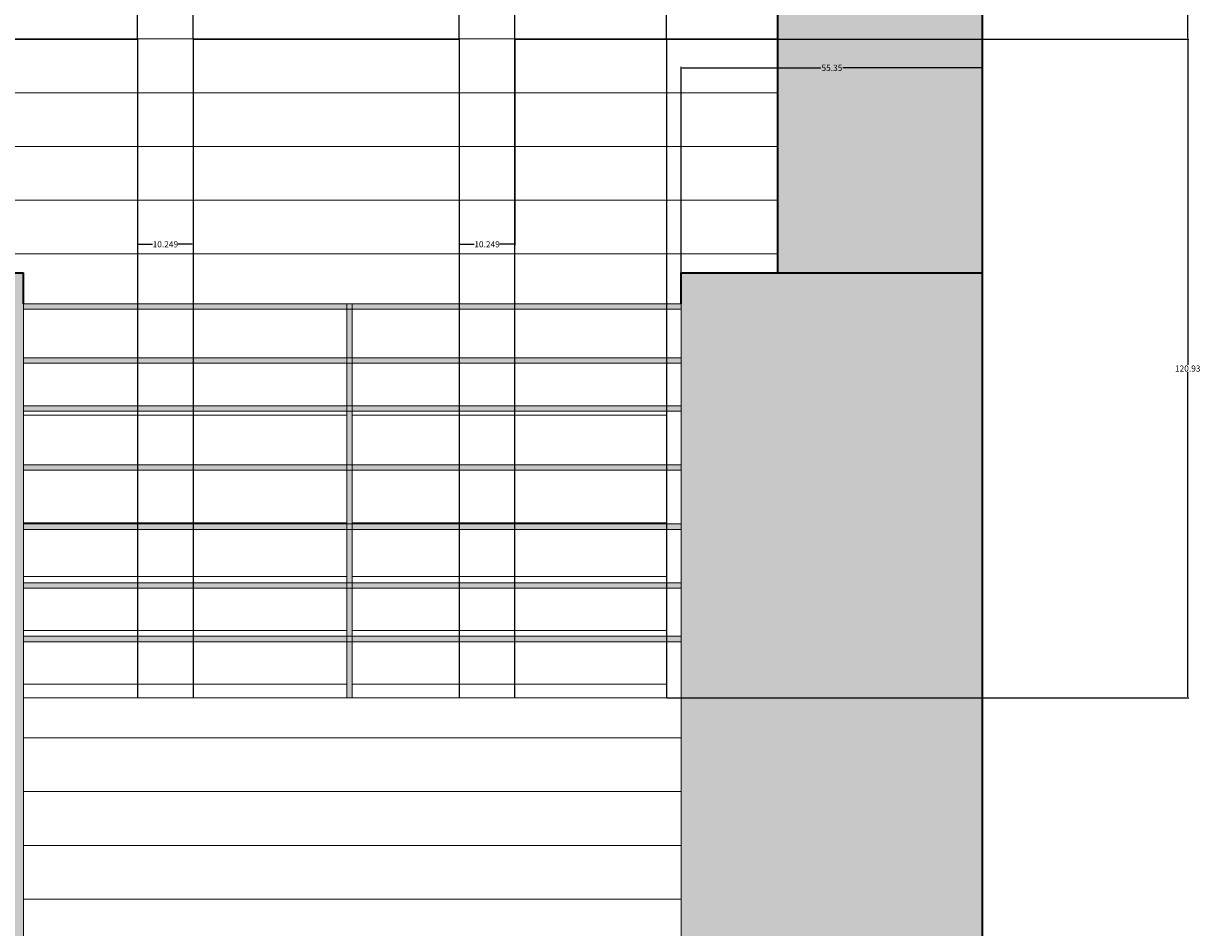
# Model space of a CAD drawing. Units: inches. Extents: x 8 to 634, y 41 to 867.
# Tile 20 of 21: x 418 to 634, y 577 to 743. Entities that reach past the tile are written whole.
import ezdxf

# ---------------------------------------------------------------- set-up
doc = ezdxf.new("R2010")
doc.units = ezdxf.units.IN
doc.header["$MEASUREMENT"] = 0
for name, color, linetype, lineweight in [('A-ANNO-DIMS', 2, 'Continuous', 18), ('A-FLOR-HRAL', 7, 'Continuous', 18), ('A-FLOR-HRAL-PATT', 252, 'Continuous', 9), ('A-GLAZ', 4, 'Continuous', 25), ('A-ROOF', 7, 'Continuous', 35), ('A-ROOF-PATT', 8, 'Continuous', 9), ('A-WALL', 7, 'Continuous', 35), ('A-WALL-PANL', 7, 'Continuous', 18), ('A-WALL-PATT', 8, 'Continuous', 9)]:
    doc.layers.add(name, color=color, linetype=linetype, lineweight=lineweight)
doc.layers.add('A-GLAZ-PATT', color=251, linetype='Continuous', lineweight=9, true_color=0x636466)
doc.styles.get("Standard").update_dxf_attribs({"font": 'arial.ttf'})
doc.dimstyles.get("Standard").update_dxf_attribs({"dimtxt": 1.125, "dimasz": 0.18, "dimexe": 0.18, "dimexo": 0.0625, "dimgap": 0.09, "dimtad": 0, "dimtih": 1, "dimtoh": 1, "dimdec": 4, "dimzin": 0, "dimdsep": 46, "dimlunit": 4, "dimtxsty": 'Standard', "dimcen": 0.09, "dimadec": 0, "dimazin": 0, "dimtfac": 1, "dimtdec": 4, "dimtofl": 0, "dimtmove": 0, "dimatfit": 3, "dimfxl": 1, "dimtolj": 1, "dimtzin": 0, "dimarcsym": 0})

# ---------------------------------------------------------------- blocks, each defined once
blk = doc.blocks.new('*D19')
at = {"layer": 'A-ANNO-DIMS', "color": 0, "lineweight": -2, "transparency": 16777216}
for p, q in [((47.34, 697.73), (47.34, 866.81)), ((47.52, 866.63), (319.51, 866.63)), ((594.17, 866.63), (322.18, 866.63)), ((594.35, 827.83), (594.35, 866.81))]:
    blk.add_line(p, q, dxfattribs=at)
at = {"layer": 'A-ANNO-DIMS', "color": 0, "transparency": 16777216}
for points in [[(47.52, 866.66), (47.52, 866.6), (47.34, 866.63)], [(594.17, 866.66), (594.17, 866.6), (594.35, 866.63)]]:
    blk.add_solid(points, dxfattribs=at)
at = {"layer": 'Defpoints', "color": 0, "transparency": 16777216}
for p in [(594.35, 866.63), (594.35, 827.77), (47.34, 697.67)]:
    blk.add_point(p, dxfattribs=at)
at = {"layer": 'A-ANNO-DIMS', "color": 0, "transparency": 16777216, "insert": (320.85, 866.63), "char_height": 1.125, "attachment_point": 5}
blk.add_mtext('\\A1;547', dxfattribs=at)
blk = doc.blocks.new('*D44')
at = {"layer": 'A-ANNO-DIMS', "color": 0, "lineweight": -2, "transparency": 16777216}
for p, q in [((536.38, 740.56), (632.18, 740.56)), ((632, 740.38), (632, 680.76)), ((632, 619.81), (632, 679.43)), ((536.38, 619.63), (632.18, 619.63))]:
    blk.add_line(p, q, dxfattribs=at)
at = {"layer": 'A-ANNO-DIMS', "color": 0, "transparency": 16777216}
for points in [[(631.97, 740.38), (632.03, 740.38), (632, 740.56)], [(631.97, 619.81), (632.03, 619.81), (632, 619.63)]]:
    blk.add_solid(points, dxfattribs=at)
at = {"layer": 'Defpoints', "color": 0, "transparency": 16777216}
for p in [(536.32, 740.56), (632, 740.56), (536.32, 619.63)]:
    blk.add_point(p, dxfattribs=at)
at = {"layer": 'A-ANNO-DIMS', "color": 0, "transparency": 16777216, "insert": (632, 680.09), "char_height": 1.125, "attachment_point": 5}
blk.add_mtext('\\A1;120.93', dxfattribs=at)
blk = doc.blocks.new('*D45')
at = {"layer": 'A-ANNO-DIMS', "color": 0, "lineweight": -2, "transparency": 16777216}
for p, q in [((556.77, 776.89), (632.18, 776.89)), ((632, 776.71), (632, 759.39)), ((632, 740.74), (632, 758.06)), ((536.38, 740.56), (632.18, 740.56))]:
    blk.add_line(p, q, dxfattribs=at)
at = {"layer": 'A-ANNO-DIMS', "color": 0, "transparency": 16777216}
for points in [[(631.97, 776.71), (632.03, 776.71), (632, 776.89)], [(631.97, 740.74), (632.03, 740.74), (632, 740.56)]]:
    blk.add_solid(points, dxfattribs=at)
at = {"layer": 'Defpoints', "color": 0, "transparency": 16777216}
for p in [(556.71, 776.89), (632, 776.89), (536.32, 740.56)]:
    blk.add_point(p, dxfattribs=at)
at = {"layer": 'A-ANNO-DIMS', "color": 0, "transparency": 16777216, "insert": (632, 758.72), "char_height": 1.125, "attachment_point": 5}
blk.add_mtext('\\A1;36.34', dxfattribs=at)
blk = doc.blocks.new('*D50')
at = {"layer": 'A-ANNO-DIMS', "color": 0, "lineweight": -2, "transparency": 16777216}
for p, q in [((370.39, 740.62), (370.39, 778.39)), ((370.57, 778.21), (402.91, 778.21)), ((439.02, 778.21), (406.68, 778.21)), ((439.2, 740.62), (439.2, 778.39))]:
    blk.add_line(p, q, dxfattribs=at)
at = {"layer": 'A-ANNO-DIMS', "color": 0, "transparency": 16777216}
for points in [[(370.57, 778.24), (370.57, 778.18), (370.39, 778.21)], [(439.02, 778.24), (439.02, 778.18), (439.2, 778.21)]]:
    blk.add_solid(points, dxfattribs=at)
at = {"layer": 'Defpoints', "color": 0, "transparency": 16777216}
for p in [(439.2, 778.21), (370.39, 740.56), (439.2, 740.56)]:
    blk.add_point(p, dxfattribs=at)
at = {"layer": 'A-ANNO-DIMS', "color": 0, "transparency": 16777216, "insert": (404.79, 778.21), "char_height": 1.125, "attachment_point": 5}
blk.add_mtext('\\A1;68.81', dxfattribs=at)
blk = doc.blocks.new('*D51')
at = {"layer": 'A-ANNO-DIMS', "color": 0, "lineweight": -2, "transparency": 16777216}
for p, q in [((439.2, 740.49), (439.2, 702.73)), ((449.45, 740.49), (449.45, 702.73)), ((439.38, 702.91), (441.95, 702.91)), ((449.27, 702.91), (446.7, 702.91))]:
    blk.add_line(p, q, dxfattribs=at)
at = {"layer": 'A-ANNO-DIMS', "color": 0, "transparency": 16777216}
for points in [[(439.38, 702.94), (439.38, 702.88), (439.2, 702.91)], [(449.27, 702.94), (449.27, 702.88), (449.45, 702.91)]]:
    blk.add_solid(points, dxfattribs=at)
at = {"layer": 'Defpoints', "color": 0, "transparency": 16777216}
for p in [(439.2, 740.56), (449.45, 740.56), (439.2, 702.91)]:
    blk.add_point(p, dxfattribs=at)
at = {"layer": 'A-ANNO-DIMS', "color": 0, "transparency": 16777216, "insert": (444.33, 702.91), "char_height": 1.125, "attachment_point": 5}
blk.add_mtext('\\A1;10.249', dxfattribs=at)
blk = doc.blocks.new('*D52')
at = {"layer": 'A-ANNO-DIMS', "color": 0, "lineweight": -2, "transparency": 16777216}
for p, q in [((449.45, 740.62), (449.45, 778.39)), ((449.63, 778.21), (472.28, 778.21)), ((498.07, 778.21), (475.43, 778.21)), ((498.25, 740.62), (498.25, 778.39))]:
    blk.add_line(p, q, dxfattribs=at)
at = {"layer": 'A-ANNO-DIMS', "color": 0, "transparency": 16777216}
for points in [[(449.63, 778.24), (449.63, 778.18), (449.45, 778.21)], [(498.07, 778.24), (498.07, 778.18), (498.25, 778.21)]]:
    blk.add_solid(points, dxfattribs=at)
at = {"layer": 'Defpoints', "color": 0, "transparency": 16777216}
for p in [(498.25, 778.21), (449.45, 740.56), (498.25, 740.56)]:
    blk.add_point(p, dxfattribs=at)
at = {"layer": 'A-ANNO-DIMS', "color": 0, "transparency": 16777216, "insert": (473.85, 778.21), "char_height": 1.125, "attachment_point": 5}
blk.add_mtext('\\A1;48.8', dxfattribs=at)
blk = doc.blocks.new('*D53')
at = {"layer": 'A-ANNO-DIMS', "color": 0, "lineweight": -2, "transparency": 16777216}
for p, q in [((498.25, 740.49), (498.25, 702.73)), ((508.5, 740.49), (508.5, 702.73)), ((498.43, 702.91), (501, 702.91)), ((508.32, 702.91), (505.75, 702.91))]:
    blk.add_line(p, q, dxfattribs=at)
at = {"layer": 'A-ANNO-DIMS', "color": 0, "transparency": 16777216}
for points in [[(498.43, 702.94), (498.43, 702.88), (498.25, 702.91)], [(508.32, 702.94), (508.32, 702.88), (508.5, 702.91)]]:
    blk.add_solid(points, dxfattribs=at)
at = {"layer": 'Defpoints', "color": 0, "transparency": 16777216}
for p in [(498.25, 740.56), (508.5, 740.56), (498.25, 702.91)]:
    blk.add_point(p, dxfattribs=at)
at = {"layer": 'A-ANNO-DIMS', "color": 0, "transparency": 16777216, "insert": (503.38, 702.91), "char_height": 1.125, "attachment_point": 5}
blk.add_mtext('\\A1;10.249', dxfattribs=at)
blk = doc.blocks.new('*D54')
at = {"layer": 'A-ANNO-DIMS', "color": 0, "lineweight": -2, "transparency": 16777216}
for p, q in [((508.5, 740.62), (508.5, 778.39)), ((508.68, 778.21), (520.42, 778.21)), ((536.14, 778.21), (524.4, 778.21)), ((536.32, 740.62), (536.32, 778.39))]:
    blk.add_line(p, q, dxfattribs=at)
at = {"layer": 'A-ANNO-DIMS', "color": 0, "transparency": 16777216}
for points in [[(508.68, 778.24), (508.68, 778.18), (508.5, 778.21)], [(536.14, 778.24), (536.14, 778.18), (536.32, 778.21)]]:
    blk.add_solid(points, dxfattribs=at)
at = {"layer": 'Defpoints', "color": 0, "transparency": 16777216}
for p in [(536.32, 778.21), (508.5, 740.56), (536.32, 740.56)]:
    blk.add_point(p, dxfattribs=at)
at = {"layer": 'A-ANNO-DIMS', "color": 0, "transparency": 16777216, "insert": (522.41, 778.21), "char_height": 1.125, "attachment_point": 5}
blk.add_mtext('\\A1;27.82', dxfattribs=at)
blk = doc.blocks.new('*D56')
at = {"layer": 'A-ANNO-DIMS', "color": 0, "lineweight": -2, "transparency": 16777216}
for p, q in [((539, 697.73), (539, 735.5)), ((539.18, 735.32), (564.68, 735.32)), ((594.17, 735.32), (568.67, 735.32)), ((594.35, 697.73), (594.35, 735.5))]:
    blk.add_line(p, q, dxfattribs=at)
at = {"layer": 'A-ANNO-DIMS', "color": 0, "transparency": 16777216}
for points in [[(539.18, 735.35), (539.18, 735.29), (539, 735.32)], [(594.17, 735.35), (594.17, 735.29), (594.35, 735.32)]]:
    blk.add_solid(points, dxfattribs=at)
at = {"layer": 'Defpoints', "color": 0, "transparency": 16777216}
for p in [(594.35, 735.32), (539, 697.67), (594.35, 697.67)]:
    blk.add_point(p, dxfattribs=at)
at = {"layer": 'A-ANNO-DIMS', "color": 0, "transparency": 16777216, "insert": (566.68, 735.32), "char_height": 1.125, "attachment_point": 5}
blk.add_mtext('\\A1;55.35', dxfattribs=at)

msp = doc.modelspace()

# ---------------------------------------------------------------- hatches: boundary and pattern name
at = {"layer": 'A-FLOR-HRAL-PATT', "transparency": 33554687}
h = msp.add_hatch(color=256, dxfattribs=at)
h.dxf.hatch_style = 1
h.paths.add_polyline_path([(439.201, 691.978), (418.2881, 691.978), (418.2881, 690.978), (439.201, 690.978)])
h.paths.add_polyline_path([(449.4498, 691.978), (439.201, 691.978), (439.201, 690.978), (449.4498, 690.978)])
h.paths.add_polyline_path([(477.6441, 691.978), (449.4498, 691.978), (449.4498, 690.978), (477.6441, 690.978)])
h.paths.add_polyline_path([(477.6441, 682.0586), (449.4498, 682.0586), (449.4498, 681.0586), (477.6441, 681.0586)])
h.paths.add_polyline_path([(449.4498, 682.0586), (439.201, 682.0586), (439.201, 681.0586), (449.4498, 681.0586)])
h.paths.add_polyline_path([(439.201, 682.0586), (418.2881, 682.0586), (418.2881, 681.0586), (439.201, 681.0586)])
h.paths.add_polyline_path([(439.201, 673.2414), (418.2881, 673.2414), (418.2881, 672.2414), (439.201, 672.2414)])
h.paths.add_polyline_path([(449.4498, 673.2414), (439.201, 673.2414), (439.201, 672.2414), (449.4498, 672.2414)])
h.paths.add_polyline_path([(539.0002, 673.2414), (449.4498, 673.2414), (449.4498, 672.2414), (539.0002, 672.2414)])
h.paths.add_polyline_path([(439.201, 662.4168), (418.2881, 662.4168), (418.2881, 661.4168), (439.201, 661.4168)], flags=16)
h.paths.add_polyline_path([(449.4498, 662.4168), (439.201, 662.4168), (439.201, 661.4168), (449.4498, 661.4168)], flags=16)
h.paths.add_polyline_path([(477.6441, 662.4168), (449.4498, 662.4168), (449.4498, 661.4168), (477.6441, 661.4168)], flags=16)
h.paths.add_polyline_path([(439.201, 651.537), (418.2881, 651.537), (418.2881, 650.537), (439.201, 650.537)])
h.paths.add_polyline_path([(449.4498, 651.537), (439.201, 651.537), (439.201, 650.537), (449.4498, 650.537)])
h.paths.add_polyline_path([(477.6441, 651.537), (449.4498, 651.537), (449.4498, 650.537), (477.6441, 650.537)])
h.paths.add_polyline_path([(439.201, 640.7358), (418.2881, 640.7358), (418.2881, 639.7358), (439.201, 639.7358)])
h.paths.add_polyline_path([(449.4498, 640.7358), (439.201, 640.7358), (439.201, 639.7358), (449.4498, 639.7358)])
h.paths.add_polyline_path([(477.6441, 640.7358), (449.4498, 640.7358), (449.4498, 639.7358), (477.6441, 639.7358)])
h.paths.add_polyline_path([(439.201, 630.9186), (418.2881, 630.9186), (418.2881, 629.9186), (439.201, 629.9186)])
h.paths.add_polyline_path([(449.4498, 630.9186), (439.201, 630.9186), (439.201, 629.9186), (449.4498, 629.9186)])
h.paths.add_polyline_path([(477.6441, 630.9186), (449.4498, 630.9186), (449.4498, 629.9186), (477.6441, 629.9186)])
h.paths.add_polyline_path([(498.2535, 630.9186), (478.6441, 630.9186), (478.6441, 629.9186), (498.2535, 629.9186)])
h.paths.add_polyline_path([(478.6441, 639.7358), (477.6441, 639.7358), (477.6441, 630.9186), (478.6441, 630.9186)])
h.paths.add_polyline_path([(478.6441, 630.9186), (477.6441, 630.9186), (477.6441, 629.9186), (478.6441, 629.9186)])
h.paths.add_polyline_path([(478.6441, 629.9186), (477.6441, 629.9186), (477.6441, 619.6298), (478.6441, 619.6298)])
h.paths.add_polyline_path([(508.5023, 630.9186), (498.2535, 630.9186), (498.2535, 629.9186), (508.5023, 629.9186)])
h.paths.add_polyline_path([(536.3204, 630.9186), (508.5023, 630.9186), (508.5023, 629.9186), (536.3204, 629.9186)])
h.paths.add_polyline_path([(539.0002, 630.9186), (536.3204, 630.9186), (536.3204, 629.9186), (539.0002, 629.9186)])
h.paths.add_polyline_path([(539.0002, 640.7358), (536.3204, 640.7358), (536.3204, 639.7358), (539.0002, 639.7358)])
h.paths.add_polyline_path([(536.3204, 640.7358), (508.5023, 640.7358), (508.5023, 639.7358), (536.3204, 639.7358)])
h.paths.add_polyline_path([(508.5023, 640.7358), (498.2535, 640.7358), (498.2535, 639.7358), (508.5023, 639.7358)])
h.paths.add_polyline_path([(498.2535, 640.7358), (478.6441, 640.7358), (478.6441, 639.7358), (498.2535, 639.7358)])
h.paths.add_polyline_path([(498.2535, 651.537), (478.6441, 651.537), (478.6441, 650.537), (498.2535, 650.537)])
h.paths.add_polyline_path([(478.6441, 651.537), (477.6441, 651.537), (477.6441, 650.537), (478.6441, 650.537)])
h.paths.add_polyline_path([(478.6441, 661.4168), (477.6441, 661.4168), (477.6441, 651.537), (478.6441, 651.537)])
h.paths.add_polyline_path([(478.6441, 650.537), (477.6441, 650.537), (477.6441, 640.7358), (478.6441, 640.7358)])
h.paths.add_polyline_path([(478.6441, 640.7358), (477.6441, 640.7358), (477.6441, 639.7358), (478.6441, 639.7358)])
h.paths.add_polyline_path([(508.5023, 651.537), (498.2535, 651.537), (498.2535, 650.537), (508.5023, 650.537)])
h.paths.add_polyline_path([(536.3204, 651.537), (508.5023, 651.537), (508.5023, 650.537), (536.3204, 650.537)])
h.paths.add_polyline_path([(539.0002, 651.537), (536.3204, 651.537), (536.3204, 650.537), (539.0002, 650.537)])
h.paths.add_polyline_path([(539.0002, 662.4168), (536.3204, 662.4168), (536.3204, 661.4168), (539.0002, 661.4168)])
h.paths.add_polyline_path([(536.3204, 662.4168), (508.5023, 662.4168), (508.5023, 661.4168), (536.3204, 661.4168)])
h.paths.add_polyline_path([(508.5023, 662.4168), (498.2535, 662.4168), (498.2535, 661.4168), (508.5023, 661.4168)])
h.paths.add_polyline_path([(498.2535, 662.4168), (418.2881, 662.4168), (418.2881, 661.4168), (498.2535, 661.4168)])
h.paths.add_polyline_path([(478.6441, 672.2414), (477.6441, 672.2414), (477.6441, 662.4168), (478.6441, 662.4168)])
h.paths.add_polyline_path([(478.6441, 681.0586), (477.6441, 681.0586), (477.6441, 673.2414), (478.6441, 673.2414)])
h = msp.add_hatch(color=256, dxfattribs=at)
h.dxf.hatch_style = 1
h.paths.add_polyline_path([(498.2535, 682.0586), (478.6441, 682.0586), (478.6441, 681.0586), (498.2535, 681.0586)])
h.paths.add_polyline_path([(508.5023, 682.0586), (498.2535, 682.0586), (498.2535, 681.0586), (508.5023, 681.0586)])
h.paths.add_polyline_path([(536.3204, 682.0586), (508.5023, 682.0586), (508.5023, 681.0586), (536.3204, 681.0586)])
h.paths.add_polyline_path([(478.6441, 690.978), (477.6441, 690.978), (477.6441, 682.0586), (478.6441, 682.0586)])
h.paths.add_polyline_path([(478.6441, 682.0586), (477.6441, 682.0586), (477.6441, 681.0586), (478.6441, 681.0586)])
h.paths.add_polyline_path([(477.6441, 662.4168), (449.4498, 662.4168), (449.4498, 661.4168), (477.6441, 661.4168)])
h.paths.add_polyline_path([(449.4498, 662.4168), (439.201, 662.4168), (439.201, 661.4168), (449.4498, 661.4168)])
h.paths.add_polyline_path([(439.201, 662.4168), (418.2881, 662.4168), (418.2881, 661.4168), (439.201, 661.4168)])
h.paths.add_polyline_path([(478.6441, 691.978), (477.6441, 691.978), (477.6441, 690.978), (478.6441, 690.978)])
h.paths.add_polyline_path([(498.2535, 691.978), (478.6441, 691.978), (478.6441, 690.978), (498.2535, 690.978)])
h.paths.add_polyline_path([(508.5023, 691.978), (498.2535, 691.978), (498.2535, 690.978), (508.5023, 690.978)])
h.paths.add_polyline_path([(536.3204, 691.978), (508.5023, 691.978), (508.5023, 690.978), (536.3204, 690.978)])
h.paths.add_polyline_path([(539.0002, 691.978), (536.3204, 691.978), (536.3204, 690.978), (539.0002, 690.978)])
h.paths.add_polyline_path([(539.0002, 682.0586), (536.3204, 682.0586), (536.3204, 681.0586), (539.0002, 681.0586)])
at = {"layer": 'A-GLAZ-PATT', "transparency": 33554687}
h = msp.add_hatch(dxfattribs=at)
h.set_pattern_fill('ANSI31', color=256, scale=79, angle=135)
h.paths.add_polyline_path([(355.7466, 740.5561), (322.56, 740.5561), (322.56, 697.6655), (355.7466, 697.6655)])
h.paths.add_polyline_path([(439.201, 740.5561), (370.3877, 740.5561), (370.3877, 697.6655), (418.2881, 697.6655), (418.2881, 691.978), (439.201, 691.978)])
h.paths.add_polyline_path([(498.2535, 740.5561), (449.4498, 740.5561), (449.4498, 691.978), (498.2535, 691.978)])
h.paths.add_polyline_path([(536.3204, 740.5561), (508.5023, 740.5561), (508.5023, 691.978), (536.3204, 691.978)])
h.paths.add_polyline_path([(439.201, 690.978), (418.2881, 690.978), (418.2881, 682.0586), (439.201, 682.0586)])
h.paths.add_polyline_path([(439.201, 681.0586), (418.2881, 681.0586), (418.2881, 673.2414), (439.201, 673.2414)])
h.paths.add_polyline_path([(439.201, 672.2414), (418.2881, 672.2414), (418.2881, 662.4168), (439.201, 662.4168)])
h.paths.add_polyline_path([(439.201, 661.4168), (418.2881, 661.4168), (418.2881, 651.537), (439.201, 651.537)])
h.paths.add_polyline_path([(439.201, 650.537), (418.2881, 650.537), (418.2881, 640.7358), (439.201, 640.7358)])
h.paths.add_polyline_path([(439.201, 639.7358), (418.2881, 639.7358), (418.2881, 630.9186), (439.201, 630.9186)])
h.paths.add_polyline_path([(439.201, 629.9186), (418.2881, 629.9186), (418.2881, 619.6298), (439.201, 619.6298)])
h.paths.add_polyline_path([(477.6441, 629.9186), (449.4498, 629.9186), (449.4498, 619.6298), (477.6441, 619.6298)])
h.paths.add_polyline_path([(477.6441, 639.7358), (449.4498, 639.7358), (449.4498, 630.9186), (477.6441, 630.9186)])
h.paths.add_polyline_path([(477.6441, 650.537), (449.4498, 650.537), (449.4498, 640.7358), (477.6441, 640.7358)])
h.paths.add_polyline_path([(477.6441, 661.4168), (449.4498, 661.4168), (449.4498, 651.537), (477.6441, 651.537)])
h.paths.add_polyline_path([(477.6441, 672.2414), (449.4498, 672.2414), (449.4498, 662.4168), (477.6441, 662.4168)])
h.paths.add_polyline_path([(477.6441, 681.0586), (449.4498, 681.0586), (449.4498, 673.2414), (477.6441, 673.2414)])
h.paths.add_polyline_path([(477.6441, 690.978), (449.4498, 690.978), (449.4498, 682.0586), (477.6441, 682.0586)])
h.paths.add_polyline_path([(498.2535, 690.978), (478.6441, 690.978), (478.6441, 682.0586), (498.2535, 682.0586)])
h.paths.add_polyline_path([(498.2535, 681.0586), (478.6441, 681.0586), (478.6441, 673.2414), (498.2535, 673.2414)])
h.paths.add_polyline_path([(498.2535, 672.2414), (478.6441, 672.2414), (478.6441, 662.4168), (498.2535, 662.4168)])
h.paths.add_polyline_path([(498.2535, 661.4168), (478.6441, 661.4168), (478.6441, 651.537), (498.2535, 651.537)])
h.paths.add_polyline_path([(498.2535, 650.537), (478.6441, 650.537), (478.6441, 640.7358), (498.2535, 640.7358)])
h.paths.add_polyline_path([(498.2535, 639.7358), (478.6441, 639.7358), (478.6441, 630.9186), (498.2535, 630.9186)])
h.paths.add_polyline_path([(498.2535, 629.9186), (478.6441, 629.9186), (478.6441, 619.6298), (498.2535, 619.6298)])
h.paths.add_polyline_path([(536.3204, 629.9186), (508.5023, 629.9186), (508.5023, 619.6298), (536.3204, 619.6298)])
h.paths.add_polyline_path([(536.3204, 639.7358), (508.5023, 639.7358), (508.5023, 630.9186), (536.3204, 630.9186)])
h.paths.add_polyline_path([(536.3204, 650.537), (508.5023, 650.537), (508.5023, 640.7358), (536.3204, 640.7358)])
h.paths.add_polyline_path([(536.3204, 661.4168), (508.5023, 661.4168), (508.5023, 651.537), (536.3204, 651.537)])
h.paths.add_polyline_path([(536.3204, 672.2414), (508.5023, 672.2414), (508.5023, 662.4168), (536.3204, 662.4168)])
h.paths.add_polyline_path([(536.3204, 681.0586), (508.5023, 681.0586), (508.5023, 673.2414), (536.3204, 673.2414)])
h.paths.add_polyline_path([(536.3204, 690.978), (508.5023, 690.978), (508.5023, 682.0586), (536.3204, 682.0586)])
h.paths.add_polyline_path([(342.6544, 175.7749), (302.6522, 224.3257), (302.6522, 101.0012), (342.6544, 149.552)])
h.paths.add_polyline_path([(342.6544, 224.3257), (302.6522, 224.3257), (342.6544, 175.7749)])
h.paths.add_polyline_path([(342.6544, 149.552), (302.6522, 101.0012), (342.6544, 101.0012)])
h.paths.add_polyline_path([(353.4573, 162.6634), (342.6544, 149.552), (342.6544, 101.0012), (353.4573, 101.0012)])
h.paths.add_polyline_path([(353.4573, 224.3257), (342.6544, 224.3257), (342.6544, 101.0012), (353.4573, 101.0012)])
h.paths.add_polyline_path([(342.6544, 175.7749), (342.6544, 149.552), (353.4573, 162.6634)], flags=17)
h = msp.add_hatch(dxfattribs=at)
h.set_pattern_fill('ANSI31', color=256, scale=79, angle=135)
h.paths.add_polyline_path([(449.4498, 690.978), (439.201, 690.978), (439.201, 682.0586), (449.4498, 682.0586)])
h.paths.add_polyline_path([(449.4498, 681.0586), (439.201, 681.0586), (439.201, 673.2414), (449.4498, 673.2414)])
h.paths.add_polyline_path([(449.4498, 672.2414), (439.201, 672.2414), (439.201, 662.4168), (449.4498, 662.4168)])
h.paths.add_polyline_path([(449.4498, 661.4168), (439.201, 661.4168), (439.201, 651.537), (449.4498, 651.537)])
h.paths.add_polyline_path([(449.4498, 650.537), (439.201, 650.537), (439.201, 640.7358), (449.4498, 640.7358)])
h.paths.add_polyline_path([(449.4498, 639.7358), (439.201, 639.7358), (439.201, 630.9186), (449.4498, 630.9186)])
h.paths.add_polyline_path([(449.4498, 629.9186), (439.201, 629.9186), (439.201, 619.6298), (449.4498, 619.6298)])
h.paths.add_polyline_path([(508.5023, 629.9186), (498.2535, 629.9186), (498.2535, 619.6298), (508.5023, 619.6298)])
h.paths.add_polyline_path([(508.5023, 639.7358), (498.2535, 639.7358), (498.2535, 630.9186), (508.5023, 630.9186)])
h.paths.add_polyline_path([(508.5023, 650.537), (498.2535, 650.537), (498.2535, 640.7358), (508.5023, 640.7358)])
h.paths.add_polyline_path([(508.5023, 661.4168), (498.2535, 661.4168), (498.2535, 651.537), (508.5023, 651.537)])
h.paths.add_polyline_path([(508.5023, 672.2414), (498.2535, 672.2414), (498.2535, 662.4168), (508.5023, 662.4168)])
h.paths.add_polyline_path([(508.5023, 681.0586), (498.2535, 681.0586), (498.2535, 673.2414), (508.5023, 673.2414)])
h.paths.add_polyline_path([(508.5023, 690.978), (498.2535, 690.978), (498.2535, 682.0586), (508.5023, 682.0586)])
at = {"layer": 'A-ROOF-PATT', "transparency": 33554687}
h = msp.add_hatch(dxfattribs=at)
h.set_pattern_fill('AR-CONC', color=256, scale=2.2, angle=135)
h.paths.add_polyline_path([(262.2266, 828.9821), (144.3564, 828.9821), (144.3564, 697.6655), (262.2266, 785.231), (245.114, 785.231), (245.114, 792.8938), (262.2266, 792.8938)])
h.paths.add_polyline_path([(594.3501, 827.7671), (262.2266, 827.7671), (262.2266, 792.8938), (262.2266, 697.6655), (299.7961, 697.6655), (299.7961, 776.8929), (556.7072, 776.8929), (556.7072, 774.3342), (556.7072, 697.6655), (594.3501, 697.6655)])
at = {"layer": 'A-WALL-PATT', "transparency": 33554687}
h = msp.add_hatch(dxfattribs=at)
h.set_pattern_fill('ANSI31', color=256, scale=79, angle=135)
h.paths.add_polyline_path([(539.0002, 276.166), (499.4677, 276.166), (418.2881, 276.166), (418.2881, 228.4951), (435.5682, 228.4951), (539.0002, 228.4951)])
h.paths.add_polyline_path([(539.0002, 228.4951), (435.5682, 228.4951), (418.2881, 228.4951), (418.2881, 112.2342), (439.3242, 112.2342), (539.0002, 112.2342)])
h.paths.add_polyline_path([(518.1129, 124.2342), (473.3277, 124.2342), (473.3277, 216.4951), (518.1129, 216.4951)], flags=16)
h.paths.add_polyline_path([(451.2116, 124.2342), (427.4368, 124.2342), (427.4368, 216.4951), (451.2116, 216.4951)], flags=16)
h.paths.add_polyline_path([(539.0002, 112.2342), (439.3242, 112.2342), (418.2881, 112.2342), (418.2881, 91.5417), (539.0002, 91.5417)])
h.paths.add_polyline_path([(539.0002, 392.4268), (427.4368, 392.4268), (418.2881, 392.4268), (418.2881, 391.7598), (418.2881, 276.166), (499.4677, 276.166), (539.0002, 276.166)])
h.paths.add_polyline_path([(518.1129, 288.166), (473.3277, 288.166), (473.3277, 380.4268), (518.1129, 380.4268)], flags=16)
h.paths.add_polyline_path([(451.2116, 288.166), (427.4368, 288.166), (427.4368, 380.4268), (451.2116, 380.4268)], flags=16)
h.paths.add_polyline_path([(539.0002, 451.6305), (427.4368, 452.9097), (418.2881, 452.9097), (418.2881, 392.4268), (427.4368, 392.4268), (539.0002, 392.4268)])
h.paths.add_polyline_path([(539.0002, 569.1705), (427.4368, 569.1705), (418.2881, 569.1705), (418.2881, 452.9097), (427.4368, 452.9097), (539.0002, 451.6305)])
h.paths.add_polyline_path([(473.3277, 557.1705), (518.1129, 557.1705), (518.1129, 464.9097), (473.3277, 464.9097)], flags=16)
h.paths.add_polyline_path([(451.2116, 557.1705), (451.2116, 464.9097), (427.4368, 464.9097), (427.4368, 557.1705)], flags=16)
h.paths.add_polyline_path([(539.0002, 619.6298), (418.2881, 619.6298), (418.2881, 569.1705), (427.4368, 569.1705), (539.0002, 569.1705)])
h.paths.add_polyline_path([(556.7072, 774.3342), (556.7072, 776.8929), (299.7961, 776.8929), (299.7961, 697.6655), (322.56, 697.6655), (322.56, 740.5561), (355.7466, 740.5561), (355.7466, 697.6655), (360.785, 697.6655), (370.3877, 697.6655), (370.3877, 740.5561), (439.201, 740.5561), (439.201, 691.978), (449.4498, 691.978), (449.4498, 740.5561), (498.2535, 740.5561), (498.2535, 691.978), (508.5023, 691.978), (508.5023, 740.5561), (536.3204, 740.5561), (536.3204, 691.978), (539.0002, 691.978), (539.0002, 697.6655), (556.7072, 697.6655)])
h = msp.add_hatch(dxfattribs=at)
h.set_pattern_fill('AR-CONC', color=256, scale=3.2)
h.paths.add_polyline_path([(119.7065, 697.6655), (47.3401, 697.6655), (47.3401, 569.1705), (119.7065, 569.1705)])
h.paths.add_polyline_path([(202.1558, 697.6655), (119.7065, 697.6655), (119.7065, 569.1705), (202.1558, 569.1705)])
h.paths.add_polyline_path([(284.6051, 697.6655), (202.1558, 697.6655), (202.1558, 569.1705), (284.6051, 569.1705)])
h.paths.add_polyline_path([(119.7065, 569.1705), (47.3401, 569.1705), (47.3401, 523.5555), (47.3401, 449.7533), (119.7065, 449.7533)])
h.paths.add_polyline_path([(342.6544, 682.1444), (360.785, 697.6655), (284.6051, 697.6655), (284.6051, 569.1705), (342.6544, 569.1705)])
h.paths.add_polyline_path([(342.6544, 569.1705), (284.6051, 569.1705), (284.6051, 449.7533), (342.6544, 449.7533)])
h.paths.add_polyline_path([(418.2881, 691.978), (418.2881, 697.6655), (360.785, 697.6655), (360.785, 569.1705), (418.2881, 569.1705)])
h.paths.add_polyline_path([(418.2881, 569.1705), (360.785, 569.1705), (360.785, 523.5555), (360.785, 449.7533), (418.2881, 449.7533)])
h.paths.add_polyline_path([(594.3501, 697.6655), (539.0002, 697.6655), (539.0002, 691.978), (539.0002, 569.1705), (594.3501, 569.1705)])
h.paths.add_polyline_path([(594.3501, 523.5555), (594.3501, 569.1705), (539.0002, 569.1705), (539.0002, 451.6305), (594.3501, 451.6305)])
h.paths.add_polyline_path([(594.3501, 451.6305), (539.0002, 451.6305), (539.0002, 391.7598), (594.3501, 391.7598)])
h.paths.add_polyline_path([(594.3501, 391.7598), (539.0002, 391.7598), (539.0002, 276.166), (594.3501, 276.166)])
h.paths.add_polyline_path([(418.2881, 449.7533), (360.785, 449.7533), (360.785, 391.7598), (418.2881, 391.7598)])
h.paths.add_polyline_path([(342.6544, 449.7533), (284.6051, 449.7533), (284.6051, 391.7598), (342.6544, 391.7598)])
h.paths.add_polyline_path([(342.6544, 391.7598), (284.6051, 391.7598), (284.6051, 272.3426), (342.6544, 272.3426)])
h.paths.add_polyline_path([(418.2881, 391.7598), (360.785, 391.7598), (360.785, 272.3426), (418.2881, 272.3426)])
h.paths.add_polyline_path([(418.2881, 272.3426), (360.785, 272.3426), (360.785, 235.5555), (418.2881, 235.5555)])
h.paths.add_polyline_path([(342.6544, 272.3426), (284.6051, 272.3426), (284.6051, 235.5555), (295.0049, 235.5555), (342.6544, 235.5555)])
h.paths.add_polyline_path([(594.3501, 276.166), (539.0002, 276.166), (539.0002, 228.4951), (594.3501, 228.4951)])
h.paths.add_polyline_path([(594.3501, 228.4951), (539.0002, 228.4951), (539.0002, 91.5417), (594.3501, 91.5417)])
h.paths.add_polyline_path([(418.2881, 235.5555), (360.785, 235.5555), (360.785, 91.5417), (418.2881, 91.5417)])
h.paths.add_polyline_path([(284.6051, 272.3426), (119.7065, 272.3426), (119.7065, 235.5555), (284.6051, 235.5555)])
h.paths.add_polyline_path([(119.7065, 272.3426), (47.3401, 272.3426), (47.3401, 235.5555), (47.3401, 91.5555), (63.5448, 91.5555), (63.5448, 227.8036), (268.998, 227.8036), (268.998, 91.5555), (295.0049, 91.5555), (295.0049, 222.583), (271.9787, 222.583), (271.9787, 229.0481), (62.4019, 229.0481), (62.4019, 222.583), (61.1827, 222.583), (61.1827, 235.5555), (119.7065, 235.5555)])
h.paths.add_polyline_path([(119.7065, 391.7598), (47.3401, 391.7598), (47.3401, 379.5555), (47.3401, 272.3426), (119.7065, 272.3426)])
h.paths.add_polyline_path([(119.7065, 449.7533), (47.3401, 449.7533), (47.3401, 391.7598), (119.7065, 391.7598)])
h.paths.add_polyline_path([(202.1558, 449.7533), (119.7065, 449.7533), (119.7065, 391.7598), (202.1558, 391.7598)])
h.paths.add_polyline_path([(284.6051, 449.7533), (202.1558, 449.7533), (202.1558, 391.7598), (284.6051, 391.7598)])

# ---------------------------------------------------------------- linework, layer by layer
at = {"layer": 'A-FLOR-HRAL'}
for p, q in [((418.2881, 691.978), (539.0002, 691.978)), ((477.6441, 619.6298), (477.6441, 691.978)), ((478.6441, 619.6298), (478.6441, 691.978)), ((418.2881, 690.978), (539.0002, 690.978)), ((418.2881, 682.0586), (539.0002, 682.0586)), ((418.2881, 681.0586), (539.0002, 681.0586)), ((418.2881, 673.2414), (539.0002, 673.2414)), ((418.2881, 672.2414), (539.0002, 672.2414)), ((418.2881, 662.4168), (539.0002, 662.4168)), ((418.2881, 661.4168), (539.0002, 661.4168)), ((418.2881, 651.537), (539.0002, 651.537)), ((418.2881, 650.537), (539.0002, 650.537)), ((418.2881, 640.7358), (539.0002, 640.7358)), ((418.2881, 639.7358), (539.0002, 639.7358)), ((418.2881, 630.9186), (539.0002, 630.9186)), ((418.2881, 629.9186), (539.0002, 629.9186)), ((418.2881, 619.6298), (539.0002, 619.6298))]:
    msp.add_line(p, q, dxfattribs=at)
at = {"layer": 'A-GLAZ'}
for p, q in [((370.3877, 740.5561), (439.201, 740.5561)), ((439.201, 740.5561), (439.201, 619.6298)), ((449.4498, 740.5561), (449.4498, 619.6298)), ((449.4498, 740.5561), (498.2535, 740.5561)), ((498.2535, 740.5561), (498.2535, 619.6298)), ((508.5023, 619.6298), (508.5023, 740.5561)), ((508.5023, 740.5561), (536.3204, 740.5561)), ((536.3204, 740.5561), (536.3204, 619.6298))]:
    msp.add_line(p, q, dxfattribs=at)
at = {"layer": 'A-ROOF'}
for p, q in [((594.3501, 697.6655), (594.3501, 827.7671)), ((556.7072, 774.3342), (556.7072, 697.6655))]:
    msp.add_line(p, q, dxfattribs=at)
at = {"layer": 'A-WALL'}
for p, q in [((360.785, 697.6655), (418.2881, 697.6655)), ((418.2881, 691.978), (418.2881, 697.6655)), ((539.0002, 691.978), (539.0002, 697.6655)), ((539.0002, 697.6655), (594.3501, 697.6655)), ((594.3501, 523.5555), (594.3501, 697.6655))]:
    msp.add_line(p, q, dxfattribs=at)
at = {"layer": 'A-WALL-PANL'}
msp.add_lwpolyline([(539.0002, 691.978), (539.0002, 91.5417), (418.2881, 91.5417), (418.2881, 691.978)], dxfattribs=at)

# ---------------------------------------------------------------- dimensions: what is measured, and where the dimension line sits
at = {"layer": 'A-ANNO-DIMS'}
for base, p1, p2, override, picture, middle in [((594.3501, 866.6321), (47.3401, 697.6655), (594.3501, 827.7671), {"dimdec": 0, "dimlfac": 1, "dimrnd": 0, "dimzin": 0, "dimdsep": 46, "dimlunit": 2}, '*D19', (320.8451, 866.6321)), ((439.201, 778.2061), (370.3877, 740.5561), (439.201, 740.5561), {"dimdec": 2, "dimlfac": 1, "dimrnd": 0, "dimzin": 0, "dimdsep": 46, "dimlunit": 2}, '*D50', (404.7943, 778.2061)), ((498.2535, 778.2061), (449.4498, 740.5561), (498.2535, 740.5561), {"dimdec": 1, "dimlfac": 1, "dimrnd": 0, "dimzin": 0, "dimdsep": 46, "dimlunit": 2}, '*D52', (473.8516, 778.2061)), ((536.3204, 778.2061), (508.5023, 740.5561), (536.3204, 740.5561), {"dimdec": 2, "dimlfac": 1, "dimrnd": 0, "dimzin": 0, "dimdsep": 46, "dimlunit": 2}, '*D54', (522.4114, 778.2061)), ((594.3501, 735.3155), (539.0002, 697.6655), (594.3501, 697.6655), {"dimdec": 2, "dimlfac": 1, "dimrnd": 0, "dimzin": 0, "dimdsep": 46, "dimlunit": 2}, '*D56', (566.6751, 735.3155))]:
    dim = msp.add_linear_dim(base=base, p1=p1, p2=p2, dimstyle='Standard', override=override, dxfattribs=at)
    dim.commit()
    dim.dimension.update_dxf_attribs({"geometry": picture, "text_midpoint": middle})
for base, p1, p2, angle, override, picture, middle in [((632.0001, 776.8929), (536.3204, 740.5561), (556.7072, 776.8929), 90, {"dimdec": 2, "dimlfac": 1, "dimrnd": 0, "dimzin": 0, "dimdsep": 46, "dimlunit": 2}, '*D45', (632.0001, 758.7245)), ((439.201, 702.9061), (449.4498, 740.5561), (439.201, 740.5561), 180, {"dimdec": 3, "dimlfac": 1, "dimrnd": 0, "dimzin": 0, "dimdsep": 46, "dimlunit": 2}, '*D51', (444.3254, 702.9061)), ((498.2535, 702.9061), (508.5023, 740.5561), (498.2535, 740.5561), 180, {"dimdec": 3, "dimlfac": 1, "dimrnd": 0, "dimzin": 0, "dimdsep": 46, "dimlunit": 2}, '*D53', (503.3779, 702.9061)), ((632.0001, 740.5561), (536.3204, 619.6298), (536.3204, 740.5561), 90, {"dimdec": 2, "dimlfac": 1, "dimrnd": 0, "dimzin": 0, "dimdsep": 46, "dimlunit": 2}, '*D44', (632.0001, 680.093))]:
    dim = msp.add_linear_dim(base=base, p1=p1, p2=p2, angle=angle, dimstyle='Standard', override=override, dxfattribs=at)
    dim.commit()
    dim.dimension.update_dxf_attribs({"geometry": picture, "text_midpoint": middle})

doc.saveas('drawing.dxf')
